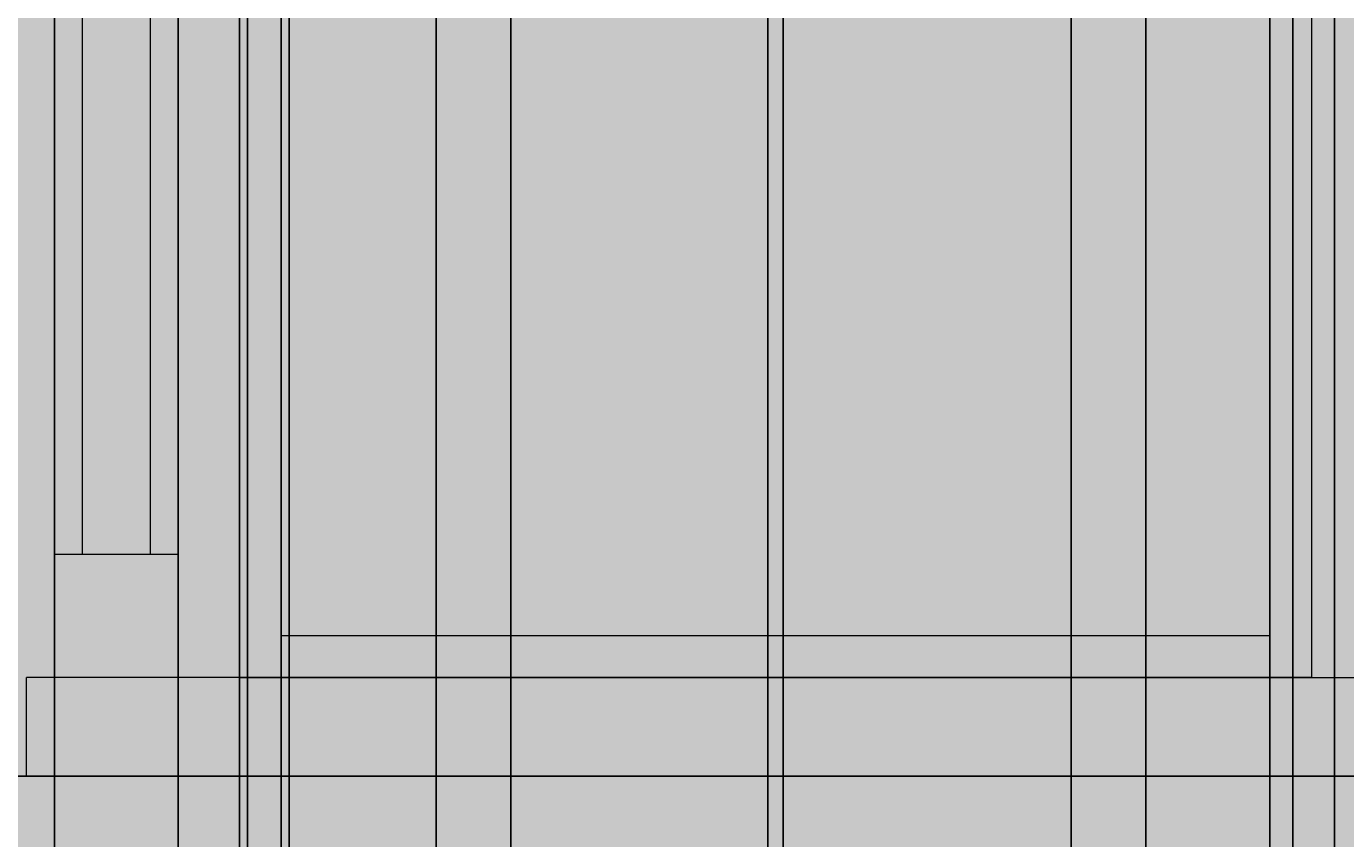
# Model space of a CAD drawing. Units: inches. Extents: x 3024 to 4744, y 1110 to 2100.
# Tile 19 of 29: x 3149 to 3275, y 1654 to 1731. Entities that reach past the tile are written whole.
import ezdxf

# ---------------------------------------------------------------- set-up
doc = ezdxf.new("R2010")
doc.units = ezdxf.units.IN
for name, color, linetype, lineweight in [('A-ANNO-DIMS', 2, 'Continuous', 18), ('A-ELEV', 7, 'Continuous', 25), ('A-ELEV-PATT', 252, 'Continuous', 13), ('A-GLAZ', 4, 'Continuous', 18)]:
    doc.layers.add(name, color=color, linetype=linetype, lineweight=lineweight)
doc.styles.get("Standard").update_dxf_attribs({"font": 'arial.ttf'})
doc.dimstyles.get("Standard").update_dxf_attribs({"dimtxt": 0.18, "dimasz": 0.18, "dimexe": 0.18, "dimexo": 0.0625, "dimgap": 0.09, "dimtad": 0, "dimtih": 1, "dimtoh": 1, "dimdec": 1, "dimzin": 0, "dimdsep": 46, "dimlunit": 3, "dimtxsty": 'Standard', "dimcen": 0.09, "dimadec": 0, "dimazin": 0, "dimtfac": 1, "dimtdec": 1, "dimtofl": 0, "dimtmove": 0, "dimatfit": 3, "dimfxl": 1, "dimtolj": 1, "dimtzin": 0, "dimarcsym": 0})

# ---------------------------------------------------------------- blocks, each defined once
blk = doc.blocks.new('WIN-BALCONY-A')
for q in [(3148.97, 1795.04), (3148.97, 1795.04), (3292.61, 1795.04), (3292.61, 1795.04)]:
    blk.add_line((3169.4, 1795.04), q)
for points in [[(3154.33, 1806.87), (3160.86, 1806.87), (3160.86, 1897.49), (3154.33, 1897.49)], [(3154.33, 1806.87), (3160.86, 1806.87), (3160.86, 1897.49), (3154.33, 1897.49)], [(3272.18, 1795.04), (3169.4, 1795.04), (3169.4, 1897.49), (3272.18, 1897.49)], [(3272.18, 1795.04), (3169.4, 1795.04), (3169.4, 1897.49), (3272.18, 1897.49)], [(3268.18, 1799.04), (3173.4, 1799.04), (3173.4, 1893.49), (3268.18, 1893.49)], [(3268.18, 1799.04), (3173.4, 1799.04), (3173.4, 1893.49), (3268.18, 1893.49)], [(3220.05, 1893.49), (3221.52, 1893.49), (3221.52, 1799.04), (3220.05, 1799.04)], [(3220.05, 1893.49), (3221.52, 1893.49), (3221.52, 1799.04), (3220.05, 1799.04)], [(3163.53, 1795.04), (3151.66, 1795.04), (3151.66, 1806.87), (3163.53, 1806.87)], [(3163.53, 1795.04), (3151.66, 1795.04), (3151.66, 1806.87), (3163.53, 1806.87)]]:
    blk.add_lwpolyline(points, close=True)
blk.add_lwpolyline([(3292.61, 1795.04), (3292.61, 1785.61), (3148.97, 1785.61), (3148.97, 1795.04)])
blk.add_lwpolyline([(3292.61, 1795.04), (3292.61, 1785.61), (3148.97, 1785.61), (3148.97, 1795.04)])
blk = doc.blocks.new('*D64')
at = {"layer": 'A-ANNO-DIMS', "color": 0, "lineweight": -2, "transparency": 16777216}
for p, q in [((3069.79, 1241.5), (3069.79, 2100.44)), ((3069.97, 2100.26), (3405.08, 2100.26)), ((3740.97, 2100.26), (3405.87, 2100.26)), ((3741.15, 1241.5), (3741.15, 2100.44))]:
    blk.add_line(p, q, dxfattribs=at)
at = {"layer": 'A-ANNO-DIMS', "color": 0, "transparency": 16777216}
for points in [[(3069.97, 2100.29), (3069.97, 2100.23), (3069.79, 2100.26)], [(3740.97, 2100.29), (3740.97, 2100.23), (3741.15, 2100.26)]]:
    blk.add_solid(points, dxfattribs=at)
at = {"layer": 'Defpoints', "color": 0, "transparency": 16777216}
for p in [(3741.15, 2100.26), (3069.79, 1241.43), (3741.15, 1241.43)]:
    blk.add_point(p, dxfattribs=at)
at = {"layer": 'A-ANNO-DIMS', "color": 0, "transparency": 16777216, "insert": (3405.47, 2100.26), "char_height": 0.18, "attachment_point": 5}
blk.add_mtext('\\A1;671.4', dxfattribs=at)
blk = doc.blocks.new('*D89')
at = {"layer": 'A-ANNO-DIMS', "color": 0, "lineweight": -2, "transparency": 16777216}
for p, q in [((3151.66, 1794.98), (3151.66, 1109.93)), ((3163.53, 1794.98), (3163.53, 1109.93)), ((3151.84, 1110.11), (3157.14, 1110.11)), ((3163.35, 1110.11), (3158.05, 1110.11))]:
    blk.add_line(p, q, dxfattribs=at)
at = {"layer": 'A-ANNO-DIMS', "color": 0, "transparency": 16777216}
for points in [[(3151.84, 1110.14), (3151.84, 1110.08), (3151.66, 1110.11)], [(3163.35, 1110.14), (3163.35, 1110.08), (3163.53, 1110.11)]]:
    blk.add_solid(points, dxfattribs=at)
at = {"layer": 'Defpoints', "color": 0, "transparency": 16777216}
for p in [(3151.66, 1795.04), (3163.53, 1795.04), (3163.53, 1110.11)]:
    blk.add_point(p, dxfattribs=at)
at = {"layer": 'A-ANNO-DIMS', "color": 0, "transparency": 16777216, "insert": (3157.59, 1110.11), "char_height": 0.18, "attachment_point": 5}
blk.add_mtext('\\A1;11.866', dxfattribs=at)
blk = doc.blocks.new('*D90')
at = {"layer": 'A-ANNO-DIMS', "color": 0, "lineweight": -2, "transparency": 16777216}
for p, q in [((3173.4, 1798.98), (3173.4, 1109.93)), ((3169.4, 1794.98), (3169.4, 1109.93)), ((3169.58, 1110.11), (3171.07, 1110.11)), ((3173.22, 1110.11), (3171.72, 1110.11))]:
    blk.add_line(p, q, dxfattribs=at)
at = {"layer": 'A-ANNO-DIMS', "color": 0, "transparency": 16777216}
for points in [[(3169.58, 1110.14), (3169.58, 1110.08), (3169.4, 1110.11)], [(3173.22, 1110.14), (3173.22, 1110.08), (3173.4, 1110.11)]]:
    blk.add_solid(points, dxfattribs=at)
at = {"layer": 'Defpoints', "color": 0, "transparency": 16777216}
for p in [(3173.4, 1799.04), (3169.4, 1795.04), (3173.4, 1110.11)]:
    blk.add_point(p, dxfattribs=at)
at = {"layer": 'A-ANNO-DIMS', "color": 0, "transparency": 16777216, "insert": (3171.4, 1110.11), "char_height": 0.18, "attachment_point": 5}
blk.add_mtext('\\A1;4.00', dxfattribs=at)
blk = doc.blocks.new('*D91')
at = {"layer": 'A-ANNO-DIMS', "color": 0, "lineweight": -2, "transparency": 16777216}
for p, q in [((3173.4, 1798.98), (3173.4, 1109.93)), ((3220.05, 1798.98), (3220.05, 1109.93)), ((3173.58, 1110.11), (3196.33, 1110.11)), ((3219.87, 1110.11), (3197.12, 1110.11))]:
    blk.add_line(p, q, dxfattribs=at)
at = {"layer": 'A-ANNO-DIMS', "color": 0, "transparency": 16777216}
for points in [[(3173.58, 1110.14), (3173.58, 1110.08), (3173.4, 1110.11)], [(3219.87, 1110.14), (3219.87, 1110.08), (3220.05, 1110.11)]]:
    blk.add_solid(points, dxfattribs=at)
at = {"layer": 'Defpoints', "color": 0, "transparency": 16777216}
for p in [(3173.4, 1799.04), (3220.05, 1799.04), (3220.05, 1110.11)]:
    blk.add_point(p, dxfattribs=at)
at = {"layer": 'A-ANNO-DIMS', "color": 0, "transparency": 16777216, "insert": (3196.72, 1110.11), "char_height": 0.18, "attachment_point": 5}
blk.add_mtext('\\A1;46.65', dxfattribs=at)
blk = doc.blocks.new('*D92')
at = {"layer": 'A-ANNO-DIMS', "color": 0, "lineweight": -2, "transparency": 16777216}
for p, q in [((3220.05, 1798.98), (3220.05, 1109.93)), ((3221.52, 1798.98), (3221.52, 1109.93)), ((3220.23, 1110.11), (3220.47, 1110.11)), ((3221.34, 1110.11), (3221.1, 1110.11))]:
    blk.add_line(p, q, dxfattribs=at)
at = {"layer": 'A-ANNO-DIMS', "color": 0, "transparency": 16777216}
for points in [[(3220.23, 1110.14), (3220.23, 1110.08), (3220.05, 1110.11)], [(3221.34, 1110.14), (3221.34, 1110.08), (3221.52, 1110.11)]]:
    blk.add_solid(points, dxfattribs=at)
at = {"layer": 'Defpoints', "color": 0, "transparency": 16777216}
for p in [(3220.05, 1799.04), (3221.52, 1799.04), (3221.52, 1110.11)]:
    blk.add_point(p, dxfattribs=at)
at = {"layer": 'A-ANNO-DIMS', "color": 0, "transparency": 16777216, "insert": (3220.79, 1110.11), "char_height": 0.18, "attachment_point": 5}
blk.add_mtext('\\A1;1.47', dxfattribs=at)
blk = doc.blocks.new('*D93')
at = {"layer": 'A-ANNO-DIMS', "color": 0, "lineweight": -2, "transparency": 16777216}
for p, q in [((3221.52, 1798.98), (3221.52, 1109.93)), ((3268.18, 1798.98), (3268.18, 1109.93)), ((3221.7, 1110.11), (3244.45, 1110.11)), ((3268, 1110.11), (3245.25, 1110.11))]:
    blk.add_line(p, q, dxfattribs=at)
at = {"layer": 'A-ANNO-DIMS', "color": 0, "transparency": 16777216}
for points in [[(3221.7, 1110.14), (3221.7, 1110.08), (3221.52, 1110.11)], [(3268, 1110.14), (3268, 1110.08), (3268.18, 1110.11)]]:
    blk.add_solid(points, dxfattribs=at)
at = {"layer": 'Defpoints', "color": 0, "transparency": 16777216}
for p in [(3221.52, 1799.04), (3268.18, 1799.04), (3268.18, 1110.11)]:
    blk.add_point(p, dxfattribs=at)
at = {"layer": 'A-ANNO-DIMS', "color": 0, "transparency": 16777216, "insert": (3244.85, 1110.11), "char_height": 0.18, "attachment_point": 5}
blk.add_mtext('\\A1;46.65', dxfattribs=at)
blk = doc.blocks.new('*D106')
at = {"layer": 'A-ANNO-DIMS', "color": 0, "lineweight": -2, "transparency": 16777216}
for p, q in [((3170.16, 1275.67), (3170.16, 2100.44)), ((3170.34, 2100.26), (3171.83, 2100.26)), ((3173.98, 2100.26), (3172.49, 2100.26)), ((3174.16, 1271.67), (3174.16, 2100.44))]:
    blk.add_line(p, q, dxfattribs=at)
at = {"layer": 'A-ANNO-DIMS', "color": 0, "transparency": 16777216}
for points in [[(3170.34, 2100.29), (3170.34, 2100.23), (3170.16, 2100.26)], [(3173.98, 2100.29), (3173.98, 2100.23), (3174.16, 2100.26)]]:
    blk.add_solid(points, dxfattribs=at)
at = {"layer": 'Defpoints', "color": 0, "transparency": 16777216}
for p in [(3174.16, 2100.26), (3170.16, 1275.61), (3174.16, 1271.61)]:
    blk.add_point(p, dxfattribs=at)
at = {"layer": 'A-ANNO-DIMS', "color": 0, "transparency": 16777216, "insert": (3172.16, 2100.26), "char_height": 0.18, "attachment_point": 5}
blk.add_mtext('\\A1;4.00', dxfattribs=at)
blk = doc.blocks.new('*D107')
at = {"layer": 'A-ANNO-DIMS', "color": 0, "lineweight": -2, "transparency": 16777216}
for p, q in [((3174.16, 1271.67), (3174.16, 2100.44)), ((3174.34, 2100.26), (3221.88, 2100.26)), ((3270.21, 2100.26), (3222.67, 2100.26)), ((3270.39, 1271.67), (3270.39, 2100.44))]:
    blk.add_line(p, q, dxfattribs=at)
at = {"layer": 'A-ANNO-DIMS', "color": 0, "transparency": 16777216}
for points in [[(3174.34, 2100.29), (3174.34, 2100.23), (3174.16, 2100.26)], [(3270.21, 2100.29), (3270.21, 2100.23), (3270.39, 2100.26)]]:
    blk.add_solid(points, dxfattribs=at)
at = {"layer": 'Defpoints', "color": 0, "transparency": 16777216}
for p in [(3270.39, 2100.26), (3174.16, 1271.61), (3270.39, 1271.61)]:
    blk.add_point(p, dxfattribs=at)
at = {"layer": 'A-ANNO-DIMS', "color": 0, "transparency": 16777216, "insert": (3222.27, 2100.26), "char_height": 0.18, "attachment_point": 5}
blk.add_mtext('\\A1;96.23', dxfattribs=at)
blk = doc.blocks.new('*D108')
at = {"layer": 'A-ANNO-DIMS', "color": 0, "lineweight": -2, "transparency": 16777216}
for p, q in [((3270.39, 1271.67), (3270.39, 2100.44)), ((3270.57, 2100.26), (3272.06, 2100.26)), ((3274.21, 2100.26), (3272.71, 2100.26)), ((3274.39, 1275.67), (3274.39, 2100.44))]:
    blk.add_line(p, q, dxfattribs=at)
at = {"layer": 'A-ANNO-DIMS', "color": 0, "transparency": 16777216}
for points in [[(3270.57, 2100.29), (3270.57, 2100.23), (3270.39, 2100.26)], [(3274.21, 2100.29), (3274.21, 2100.23), (3274.39, 2100.26)]]:
    blk.add_solid(points, dxfattribs=at)
at = {"layer": 'Defpoints', "color": 0, "transparency": 16777216}
for p in [(3274.39, 2100.26), (3274.39, 1275.61), (3270.39, 1271.61)]:
    blk.add_point(p, dxfattribs=at)
at = {"layer": 'A-ANNO-DIMS', "color": 0, "transparency": 16777216, "insert": (3272.39, 2100.26), "char_height": 0.18, "attachment_point": 5}
blk.add_mtext('\\A1;4.00', dxfattribs=at)
blk = doc.blocks.new('*D124')
at = {"layer": 'A-ANNO-DIMS', "color": 0, "lineweight": -2, "transparency": 16777216}
for p, q in [((3174.16, 1271.67), (3174.16, 2100.44)), ((3174.34, 2100.26), (3180.75, 2100.26)), ((3188.08, 2100.26), (3181.67, 2100.26)), ((3188.26, 1256.29), (3188.26, 2100.44))]:
    blk.add_line(p, q, dxfattribs=at)
at = {"layer": 'A-ANNO-DIMS', "color": 0, "transparency": 16777216}
for points in [[(3174.34, 2100.29), (3174.34, 2100.23), (3174.16, 2100.26)], [(3188.08, 2100.29), (3188.08, 2100.23), (3188.26, 2100.26)]]:
    blk.add_solid(points, dxfattribs=at)
at = {"layer": 'Defpoints', "color": 0, "transparency": 16777216}
for p in [(3188.26, 2100.26), (3174.16, 1271.61), (3188.26, 1256.23)]:
    blk.add_point(p, dxfattribs=at)
at = {"layer": 'A-ANNO-DIMS', "color": 0, "transparency": 16777216, "insert": (3181.21, 2100.26), "char_height": 0.18, "attachment_point": 5}
blk.add_mtext('\\A1;14.098', dxfattribs=at)
blk = doc.blocks.new('*D125')
at = {"layer": 'A-ANNO-DIMS', "color": 0, "lineweight": -2, "transparency": 16777216}
for p, q in [((3188.26, 1256.29), (3188.26, 2100.44)), ((3188.44, 2100.26), (3191.44, 2100.26)), ((3195.23, 2100.26), (3192.22, 2100.26)), ((3195.41, 1256.29), (3195.41, 2100.44))]:
    blk.add_line(p, q, dxfattribs=at)
at = {"layer": 'A-ANNO-DIMS', "color": 0, "transparency": 16777216}
for points in [[(3188.44, 2100.29), (3188.44, 2100.23), (3188.26, 2100.26)], [(3195.23, 2100.29), (3195.23, 2100.23), (3195.41, 2100.26)]]:
    blk.add_solid(points, dxfattribs=at)
at = {"layer": 'Defpoints', "color": 0, "transparency": 16777216}
for p in [(3195.41, 2100.26), (3188.26, 1256.23), (3195.41, 1256.23)]:
    blk.add_point(p, dxfattribs=at)
at = {"layer": 'A-ANNO-DIMS', "color": 0, "transparency": 16777216, "insert": (3191.83, 2100.26), "char_height": 0.18, "attachment_point": 5}
blk.add_mtext('\\A1;7.147', dxfattribs=at)
blk = doc.blocks.new('*D126')
at = {"layer": 'A-ANNO-DIMS', "color": 0, "lineweight": -2, "transparency": 16777216}
for p, q in [((3249.14, 1256.29), (3249.14, 2100.44)), ((3249.32, 2100.26), (3252.32, 2100.26)), ((3256.11, 2100.26), (3253.11, 2100.26)), ((3256.29, 1256.29), (3256.29, 2100.44))]:
    blk.add_line(p, q, dxfattribs=at)
at = {"layer": 'A-ANNO-DIMS', "color": 0, "transparency": 16777216}
for points in [[(3249.32, 2100.29), (3249.32, 2100.23), (3249.14, 2100.26)], [(3256.11, 2100.29), (3256.11, 2100.23), (3256.29, 2100.26)]]:
    blk.add_solid(points, dxfattribs=at)
at = {"layer": 'Defpoints', "color": 0, "transparency": 16777216}
for p in [(3256.29, 2100.26), (3249.14, 1256.23), (3256.29, 1256.23)]:
    blk.add_point(p, dxfattribs=at)
at = {"layer": 'A-ANNO-DIMS', "color": 0, "transparency": 16777216, "insert": (3252.72, 2100.26), "char_height": 0.18, "attachment_point": 5}
blk.add_mtext('\\A1;7.147', dxfattribs=at)

msp = doc.modelspace()

# ---------------------------------------------------------------- hatches: boundary and pattern name
at = {"layer": 'A-ELEV-PATT'}
h = msp.add_hatch(color=256, dxfattribs=at)
h.dxf.hatch_style = 1
h.paths.add_polyline_path([(3491.8271, 2054.7584), (3320.5658, 2054.7584), (3320.5658, 2043.5286), (3491.8271, 2043.5286)])
h.paths.add_polyline_path([(3292.6051, 1905.6112), (3148.9694, 1905.6112), (3148.9694, 1897.4879), (3169.3964, 1897.4879), (3292.6051, 1897.4879)])
h.paths.add_polyline_path([(3292.6051, 1795.0431), (3169.3964, 1795.0431), (3148.9694, 1795.0431), (3148.9694, 1785.6112), (3292.6051, 1785.6112)])
h.paths.add_polyline_path([(3292.6051, 1779.6112), (3148.9694, 1779.6112), (3148.9694, 1771.4879), (3169.3964, 1771.4879), (3292.6051, 1771.4879)])
h.paths.add_polyline_path([(3292.6051, 1669.0431), (3169.3964, 1669.0431), (3148.9694, 1669.0431), (3148.9694, 1659.6112), (3292.6051, 1659.6112)])
h.paths.add_polyline_path([(3292.6051, 1653.6112), (3148.9694, 1653.6112), (3148.9694, 1645.4879), (3169.3964, 1645.4879), (3292.6051, 1645.4879)])
h.paths.add_polyline_path([(3292.6051, 1543.0431), (3169.3964, 1543.0431), (3148.9694, 1543.0431), (3148.9694, 1533.6112), (3292.6051, 1533.6112)])
h.paths.add_polyline_path([(3292.6051, 1527.6112), (3148.9694, 1527.6112), (3148.9694, 1519.4879), (3169.3964, 1519.4879), (3292.6051, 1519.4879)])
h.paths.add_polyline_path([(3292.6051, 1401.6112), (3148.9694, 1401.6112), (3148.9694, 1393.4879), (3169.3964, 1393.4879), (3292.6051, 1393.4879)])
h.paths.add_polyline_path([(3292.6051, 1417.0431), (3169.3964, 1417.0431), (3148.9694, 1417.0431), (3148.9694, 1407.6112), (3292.6051, 1407.6112)])
h.paths.add_polyline_path([(3292.6051, 1291.0431), (3169.3964, 1291.0431), (3148.9694, 1291.0431), (3148.9694, 1281.6112), (3292.6051, 1281.6112)])
h.paths.add_polyline_path([(3654.037, 1165.0431), (3530.8283, 1165.0431), (3510.4013, 1165.0431), (3510.4013, 1155.6112), (3654.037, 1155.6112)])
h.paths.add_polyline_path([(3654.037, 1275.6112), (3510.4013, 1275.6112), (3510.4013, 1267.4879), (3530.8283, 1267.4879), (3654.037, 1267.4879)])
h.paths.add_polyline_path([(3654.037, 1291.0431), (3530.8283, 1291.0431), (3510.4013, 1291.0431), (3510.4013, 1281.6112), (3654.037, 1281.6112)])
h.paths.add_polyline_path([(3654.037, 1417.0431), (3530.8283, 1417.0431), (3510.4013, 1417.0431), (3510.4013, 1407.6112), (3654.037, 1407.6112)])
h.paths.add_polyline_path([(3654.037, 1401.6112), (3510.4013, 1401.6112), (3510.4013, 1393.4879), (3530.8283, 1393.4879), (3654.037, 1393.4879)])
h.paths.add_polyline_path([(3654.037, 1543.0431), (3530.8283, 1543.0431), (3510.4013, 1543.0431), (3510.4013, 1533.6112), (3654.037, 1533.6112)])
h.paths.add_polyline_path([(3654.037, 1527.6112), (3510.4013, 1527.6112), (3510.4013, 1519.4879), (3530.8283, 1519.4879), (3654.037, 1519.4879)])
h.paths.add_polyline_path([(3654.037, 1653.6112), (3510.4013, 1653.6112), (3510.4013, 1645.4879), (3530.8283, 1645.4879), (3654.037, 1645.4879)])
h.paths.add_polyline_path([(3654.037, 1669.0431), (3530.8283, 1669.0431), (3510.4013, 1669.0431), (3510.4013, 1659.6112), (3654.037, 1659.6112)])
h.paths.add_polyline_path([(3654.037, 1779.6112), (3510.4013, 1779.6112), (3510.4013, 1771.4879), (3530.8283, 1771.4879), (3654.037, 1771.4879)])
h.paths.add_polyline_path([(3654.037, 1795.0431), (3530.8283, 1795.0431), (3510.4013, 1795.0431), (3510.4013, 1785.6112), (3654.037, 1785.6112)])
h.paths.add_polyline_path([(3654.037, 1905.6112), (3510.4013, 1905.6112), (3510.4013, 1897.4879), (3530.8283, 1897.4879), (3654.037, 1897.4879)])
h = msp.add_hatch(color=256, dxfattribs=at)
h.dxf.hatch_style = 1
h.paths.add_polyline_path([(3329.7033, 1407.6112), (3105.4722, 1407.6112), (3105.4722, 1401.6112), (3329.7033, 1401.6112)])
h.paths.add_polyline_path([(3329.7033, 1281.6112), (3105.4722, 1281.6112), (3105.4722, 1275.6112), (3112.3838, 1275.6112), (3329.7033, 1275.6112)])
h.paths.add_polyline_path([(3329.7033, 1533.6112), (3105.4722, 1533.6112), (3105.4722, 1527.6112), (3329.7033, 1527.6112)])
h.paths.add_polyline_path([(3329.7033, 1659.6112), (3105.4722, 1659.6112), (3105.4722, 1653.6112), (3329.7033, 1653.6112)])
h.paths.add_polyline_path([(3329.7033, 1785.6112), (3105.4722, 1785.6112), (3105.4722, 1779.6112), (3329.7033, 1779.6112)])
h.paths.add_polyline_path([(3329.7033, 1911.6112), (3105.4722, 1911.6112), (3095.7158, 1911.6112), (3095.7158, 1905.6112), (3329.7033, 1905.6112)])
h.paths.add_polyline_path([(3715.2286, 1911.6112), (3705.4722, 1911.6112), (3705.4722, 1905.6112), (3715.2286, 1905.6112)])
h.paths.add_polyline_path([(3688.5588, 1911.6112), (3481.2411, 1911.6112), (3481.2411, 1905.6112), (3688.5588, 1905.6112)])
h = msp.add_hatch(color=256, dxfattribs=at)
h.dxf.hatch_style = 1
h.paths.add_polyline_path([(3154.3287, 1897.4879), (3148.9694, 1897.4879), (3148.9694, 1905.6112), (3105.4722, 1905.6112), (3105.4722, 1785.6112), (3148.9694, 1785.6112), (3148.9694, 1795.0431), (3151.6604, 1795.0431), (3151.6604, 1806.8674), (3154.3287, 1806.8674)])
h.paths.add_polyline_path([(3329.7033, 1905.6112), (3292.6051, 1905.6112), (3292.6051, 1897.4879), (3287.2458, 1897.4879), (3287.2458, 1806.8674), (3288.3759, 1806.8674), (3288.3759, 1795.0431), (3292.6051, 1795.0431), (3292.6051, 1785.6112), (3329.7033, 1785.6112)])
h.paths.add_polyline_path([(3154.3287, 1771.4879), (3148.9694, 1771.4879), (3148.9694, 1779.6112), (3105.4722, 1779.6112), (3105.4722, 1659.6112), (3148.9694, 1659.6112), (3148.9694, 1669.0431), (3151.6604, 1669.0431), (3151.6604, 1680.8674), (3154.3287, 1680.8674)])
h.paths.add_polyline_path([(3329.7033, 1779.6112), (3292.6051, 1779.6112), (3292.6051, 1771.4879), (3287.2458, 1771.4879), (3287.2458, 1680.8674), (3288.3759, 1680.8674), (3288.3759, 1669.0431), (3292.6051, 1669.0431), (3292.6051, 1659.6112), (3329.7033, 1659.6112)])
h.paths.add_polyline_path([(3154.3287, 1645.4879), (3148.9694, 1645.4879), (3148.9694, 1653.6112), (3105.4722, 1653.6112), (3105.4722, 1533.6112), (3148.9694, 1533.6112), (3148.9694, 1543.0431), (3151.6604, 1543.0431), (3151.6604, 1554.8674), (3154.3287, 1554.8674)])
h.paths.add_polyline_path([(3329.7033, 1653.6112), (3292.6051, 1653.6112), (3292.6051, 1645.4879), (3287.2458, 1645.4879), (3287.2458, 1554.8674), (3288.3759, 1554.8674), (3288.3759, 1543.0431), (3292.6051, 1543.0431), (3292.6051, 1533.6112), (3329.7033, 1533.6112)])
h.paths.add_polyline_path([(3329.7033, 1527.6112), (3292.6051, 1527.6112), (3292.6051, 1519.4879), (3287.2458, 1519.4879), (3287.2458, 1428.8674), (3288.3759, 1428.8674), (3288.3759, 1417.0431), (3292.6051, 1417.0431), (3292.6051, 1407.6112), (3329.7033, 1407.6112)])
h.paths.add_polyline_path([(3329.7033, 1401.6112), (3292.6051, 1401.6112), (3292.6051, 1393.4879), (3287.2458, 1393.4879), (3287.2458, 1302.8674), (3288.3759, 1302.8674), (3288.3759, 1291.0431), (3292.6051, 1291.0431), (3292.6051, 1281.6112), (3329.7033, 1281.6112)])
h.paths.add_polyline_path([(3154.3287, 1393.4879), (3148.9694, 1393.4879), (3148.9694, 1401.6112), (3105.4722, 1401.6112), (3105.4722, 1281.6112), (3148.9694, 1281.6112), (3148.9694, 1291.0431), (3151.6604, 1291.0431), (3151.6604, 1302.8674), (3154.3287, 1302.8674)])
h.paths.add_polyline_path([(3154.3287, 1519.4879), (3148.9694, 1519.4879), (3148.9694, 1527.6112), (3105.4722, 1527.6112), (3105.4722, 1407.6112), (3148.9694, 1407.6112), (3148.9694, 1417.0431), (3151.6604, 1417.0431), (3151.6604, 1428.8674), (3154.3287, 1428.8674)])
h.paths.add_polyline_path([(3515.7606, 1897.4879), (3510.4013, 1897.4879), (3510.4013, 1905.6112), (3481.2411, 1905.6112), (3481.2411, 1785.6112), (3510.4013, 1785.6112), (3510.4013, 1795.0431), (3513.0923, 1795.0431), (3513.0923, 1806.8674), (3515.7606, 1806.8674)])
h.paths.add_polyline_path([(3688.5588, 1905.6112), (3654.037, 1905.6112), (3654.037, 1897.4879), (3648.6777, 1897.4879), (3648.6777, 1806.8674), (3649.8078, 1806.8674), (3649.8078, 1795.0431), (3654.037, 1795.0431), (3654.037, 1785.6112), (3688.5588, 1785.6112)])
h.paths.add_polyline_path([(3515.7606, 1771.4879), (3510.4013, 1771.4879), (3510.4013, 1779.6112), (3481.2411, 1779.6112), (3481.2411, 1659.6112), (3510.4013, 1659.6112), (3510.4013, 1669.0431), (3513.0923, 1669.0431), (3513.0923, 1680.8674), (3515.7606, 1680.8674)])
h.paths.add_polyline_path([(3688.5588, 1779.6112), (3654.037, 1779.6112), (3654.037, 1771.4879), (3648.6777, 1771.4879), (3648.6777, 1680.8674), (3649.8078, 1680.8674), (3649.8078, 1669.0431), (3654.037, 1669.0431), (3654.037, 1659.6112), (3688.5588, 1659.6112)])
h.paths.add_polyline_path([(3515.7606, 1645.4879), (3510.4013, 1645.4879), (3510.4013, 1653.6112), (3481.2411, 1653.6112), (3481.2411, 1533.6112), (3510.4013, 1533.6112), (3510.4013, 1543.0431), (3513.0923, 1543.0431), (3513.0923, 1554.8674), (3515.7606, 1554.8674)])
h.paths.add_polyline_path([(3688.5588, 1653.6112), (3654.037, 1653.6112), (3654.037, 1645.4879), (3648.6777, 1645.4879), (3648.6777, 1554.8674), (3649.8078, 1554.8674), (3649.8078, 1543.0431), (3654.037, 1543.0431), (3654.037, 1533.6112), (3688.5588, 1533.6112)])
h.paths.add_polyline_path([(3515.7606, 1519.4879), (3510.4013, 1519.4879), (3510.4013, 1527.6112), (3481.2411, 1527.6112), (3481.2411, 1407.6112), (3510.4013, 1407.6112), (3510.4013, 1417.0431), (3513.0923, 1417.0431), (3513.0923, 1428.8674), (3515.7606, 1428.8674)])
h.paths.add_polyline_path([(3688.5588, 1527.6112), (3654.037, 1527.6112), (3654.037, 1519.4879), (3648.6777, 1519.4879), (3648.6777, 1428.8674), (3649.8078, 1428.8674), (3649.8078, 1417.0431), (3654.037, 1417.0431), (3654.037, 1407.6112), (3688.5588, 1407.6112)])
h.paths.add_polyline_path([(3515.7606, 1393.4879), (3510.4013, 1393.4879), (3510.4013, 1401.6112), (3481.2411, 1401.6112), (3481.2411, 1281.6112), (3510.4013, 1281.6112), (3510.4013, 1291.0431), (3513.0923, 1291.0431), (3513.0923, 1302.8674), (3515.7606, 1302.8674)])
h.paths.add_polyline_path([(3688.5588, 1401.6112), (3654.037, 1401.6112), (3654.037, 1393.4879), (3648.6777, 1393.4879), (3648.6777, 1302.8674), (3649.8078, 1302.8674), (3649.8078, 1291.0431), (3654.037, 1291.0431), (3654.037, 1281.6112), (3688.5588, 1281.6112)])
h.paths.add_polyline_path([(3515.7606, 1267.4879), (3510.4013, 1267.4879), (3510.4013, 1275.6112), (3481.2411, 1275.6112), (3481.2411, 1155.6112), (3510.4013, 1155.6112), (3510.4013, 1165.0431), (3513.0923, 1165.0431), (3513.0923, 1176.8674), (3515.7606, 1176.8674)])
h.paths.add_polyline_path([(3688.5588, 1275.6112), (3654.037, 1275.6112), (3654.037, 1267.4879), (3648.6777, 1267.4879), (3648.6777, 1176.8674), (3649.8078, 1176.8674), (3649.8078, 1165.0431), (3654.037, 1165.0431), (3654.037, 1155.6112), (3688.5588, 1155.6112)])
h.paths.add_polyline_path([(3112.3838, 1275.6112), (3105.4722, 1275.6112), (3105.4722, 1171.0239), (3112.3838, 1171.0239)])
h = msp.add_hatch(color=256, dxfattribs=at)
h.dxf.hatch_style = 1
h.paths.add_polyline_path([(3160.8586, 1897.4879), (3154.3287, 1897.4879), (3154.3287, 1806.8674), (3160.8586, 1806.8674)])
h.paths.add_polyline_path([(3287.2458, 1897.4879), (3280.716, 1897.4879), (3280.716, 1806.8674), (3287.2458, 1806.8674)])
h.paths.add_polyline_path([(3160.8586, 1771.4879), (3154.3287, 1771.4879), (3154.3287, 1680.8674), (3160.8586, 1680.8674)])
h.paths.add_polyline_path([(3287.2458, 1771.4879), (3280.716, 1771.4879), (3280.716, 1680.8674), (3287.2458, 1680.8674)])
h.paths.add_polyline_path([(3160.8586, 1645.4879), (3154.3287, 1645.4879), (3154.3287, 1554.8674), (3160.8586, 1554.8674)])
h.paths.add_polyline_path([(3287.2458, 1645.4879), (3280.716, 1645.4879), (3280.716, 1554.8674), (3287.2458, 1554.8674)])
h.paths.add_polyline_path([(3160.8586, 1519.4879), (3154.3287, 1519.4879), (3154.3287, 1428.8674), (3160.8586, 1428.8674)])
h.paths.add_polyline_path([(3287.2458, 1519.4879), (3280.716, 1519.4879), (3280.716, 1428.8674), (3287.2458, 1428.8674)])
h.paths.add_polyline_path([(3160.8586, 1393.4879), (3154.3287, 1393.4879), (3154.3287, 1302.8674), (3160.8586, 1302.8674)])
h.paths.add_polyline_path([(3287.2458, 1393.4879), (3280.716, 1393.4879), (3280.716, 1302.8674), (3287.2458, 1302.8674)])
h.paths.add_polyline_path([(3648.6777, 1267.4879), (3642.1479, 1267.4879), (3642.1479, 1176.8674), (3648.6777, 1176.8674)])
h.paths.add_polyline_path([(3522.2905, 1267.4879), (3515.7606, 1267.4879), (3515.7606, 1176.8674), (3522.2905, 1176.8674)])
h.paths.add_polyline_path([(3522.2905, 1393.4879), (3515.7606, 1393.4879), (3515.7606, 1302.8674), (3522.2905, 1302.8674)])
h.paths.add_polyline_path([(3648.6777, 1393.4879), (3642.1479, 1393.4879), (3642.1479, 1302.8674), (3648.6777, 1302.8674)])
h.paths.add_polyline_path([(3522.2905, 1519.4879), (3515.7606, 1519.4879), (3515.7606, 1428.8674), (3522.2905, 1428.8674)])
h.paths.add_polyline_path([(3648.6777, 1519.4879), (3642.1479, 1519.4879), (3642.1479, 1428.8674), (3648.6777, 1428.8674)])
h.paths.add_polyline_path([(3522.2905, 1645.4879), (3515.7606, 1645.4879), (3515.7606, 1554.8674), (3522.2905, 1554.8674)])
h.paths.add_polyline_path([(3522.2905, 1771.4879), (3515.7606, 1771.4879), (3515.7606, 1680.8674), (3522.2905, 1680.8674)])
h.paths.add_polyline_path([(3648.6777, 1645.4879), (3642.1479, 1645.4879), (3642.1479, 1554.8674), (3648.6777, 1554.8674)])
h.paths.add_polyline_path([(3648.6777, 1771.4879), (3642.1479, 1771.4879), (3642.1479, 1680.8674), (3648.6777, 1680.8674)])
h.paths.add_polyline_path([(3648.6777, 1897.4879), (3642.1479, 1897.4879), (3642.1479, 1806.8674), (3648.6777, 1806.8674)])
h.paths.add_polyline_path([(3522.2905, 1897.4879), (3515.7606, 1897.4879), (3515.7606, 1806.8674), (3522.2905, 1806.8674)])
h = msp.add_hatch(color=256, dxfattribs=at)
h.dxf.hatch_style = 1
h.paths.add_polyline_path([(3169.3964, 1897.4879), (3160.8586, 1897.4879), (3160.8586, 1806.8674), (3163.5269, 1806.8674), (3163.5269, 1795.0431), (3169.3964, 1795.0431)])
h.paths.add_polyline_path([(3280.716, 1897.4879), (3272.1781, 1897.4879), (3272.1781, 1795.0431), (3276.5094, 1795.0431), (3276.5094, 1806.8674), (3280.716, 1806.8674)])
h.paths.add_polyline_path([(3280.716, 1771.4879), (3272.1781, 1771.4879), (3272.1781, 1669.0431), (3276.5094, 1669.0431), (3276.5094, 1680.8674), (3280.716, 1680.8674)])
h.paths.add_polyline_path([(3169.3964, 1771.4879), (3160.8586, 1771.4879), (3160.8586, 1680.8674), (3163.5269, 1680.8674), (3163.5269, 1669.0431), (3169.3964, 1669.0431)])
h.paths.add_polyline_path([(3169.3964, 1645.4879), (3160.8586, 1645.4879), (3160.8586, 1554.8674), (3163.5269, 1554.8674), (3163.5269, 1543.0431), (3169.3964, 1543.0431)])
h.paths.add_polyline_path([(3280.716, 1645.4879), (3272.1781, 1645.4879), (3272.1781, 1543.0431), (3276.5094, 1543.0431), (3276.5094, 1554.8674), (3280.716, 1554.8674)])
h.paths.add_polyline_path([(3169.3964, 1519.4879), (3160.8586, 1519.4879), (3160.8586, 1428.8674), (3163.5269, 1428.8674), (3163.5269, 1417.0431), (3169.3964, 1417.0431)])
h.paths.add_polyline_path([(3280.716, 1519.4879), (3272.1781, 1519.4879), (3272.1781, 1417.0431), (3276.5094, 1417.0431), (3276.5094, 1428.8674), (3280.716, 1428.8674)])
h.paths.add_polyline_path([(3169.3964, 1393.4879), (3160.8586, 1393.4879), (3160.8586, 1302.8674), (3163.5269, 1302.8674), (3163.5269, 1291.0431), (3169.3964, 1291.0431)])
h.paths.add_polyline_path([(3280.716, 1393.4879), (3272.1781, 1393.4879), (3272.1781, 1291.0431), (3276.5094, 1291.0431), (3276.5094, 1302.8674), (3280.716, 1302.8674)])
h.paths.add_polyline_path([(3642.1479, 1267.4879), (3633.61, 1267.4879), (3633.61, 1165.0431), (3637.9413, 1165.0431), (3637.9413, 1176.8674), (3642.1479, 1176.8674)])
h.paths.add_polyline_path([(3530.8283, 1267.4879), (3522.2905, 1267.4879), (3522.2905, 1176.8674), (3524.9588, 1176.8674), (3524.9588, 1165.0431), (3530.8283, 1165.0431)])
h.paths.add_polyline_path([(3642.1479, 1393.4879), (3633.61, 1393.4879), (3633.61, 1291.0431), (3637.9413, 1291.0431), (3637.9413, 1302.8674), (3642.1479, 1302.8674)])
h.paths.add_polyline_path([(3530.8283, 1393.4879), (3522.2905, 1393.4879), (3522.2905, 1302.8674), (3524.9588, 1302.8674), (3524.9588, 1291.0431), (3530.8283, 1291.0431)])
h.paths.add_polyline_path([(3530.8283, 1519.4879), (3522.2905, 1519.4879), (3522.2905, 1428.8674), (3524.9588, 1428.8674), (3524.9588, 1417.0431), (3530.8283, 1417.0431)])
h.paths.add_polyline_path([(3642.1479, 1519.4879), (3633.61, 1519.4879), (3633.61, 1417.0431), (3637.9413, 1417.0431), (3637.9413, 1428.8674), (3642.1479, 1428.8674)])
h.paths.add_polyline_path([(3530.8283, 1645.4879), (3522.2905, 1645.4879), (3522.2905, 1554.8674), (3524.9588, 1554.8674), (3524.9588, 1543.0431), (3530.8283, 1543.0431)])
h.paths.add_polyline_path([(3642.1479, 1645.4879), (3633.61, 1645.4879), (3633.61, 1543.0431), (3637.9413, 1543.0431), (3637.9413, 1554.8674), (3642.1479, 1554.8674)])
h.paths.add_polyline_path([(3642.1479, 1771.4879), (3633.61, 1771.4879), (3633.61, 1669.0431), (3637.9413, 1669.0431), (3637.9413, 1680.8674), (3642.1479, 1680.8674)])
h.paths.add_polyline_path([(3530.8283, 1771.4879), (3522.2905, 1771.4879), (3522.2905, 1680.8674), (3524.9588, 1680.8674), (3524.9588, 1669.0431), (3530.8283, 1669.0431)])
h.paths.add_polyline_path([(3530.8283, 1897.4879), (3522.2905, 1897.4879), (3522.2905, 1806.8674), (3524.9588, 1806.8674), (3524.9588, 1795.0431), (3530.8283, 1795.0431)])
h.paths.add_polyline_path([(3642.1479, 1897.4879), (3633.61, 1897.4879), (3633.61, 1795.0431), (3637.9413, 1795.0431), (3637.9413, 1806.8674), (3642.1479, 1806.8674)])
h = msp.add_hatch(color=256, dxfattribs=at)
h.dxf.hatch_style = 1
h.paths.add_polyline_path([(3220.0505, 1893.4879), (3173.3964, 1893.4879), (3173.3964, 1799.0431), (3220.0505, 1799.0431)])
h.paths.add_polyline_path([(3268.1781, 1893.4879), (3221.5241, 1893.4879), (3221.5241, 1799.0431), (3268.1781, 1799.0431)])
h.paths.add_polyline_path([(3581.4824, 1893.4879), (3534.8283, 1893.4879), (3534.8283, 1799.0431), (3581.4824, 1799.0431)])
h.paths.add_polyline_path([(3629.61, 1893.4879), (3582.956, 1893.4879), (3582.956, 1799.0431), (3629.61, 1799.0431)])
h.paths.add_polyline_path([(3581.4824, 1767.4879), (3534.8283, 1767.4879), (3534.8283, 1673.0431), (3581.4824, 1673.0431)])
h.paths.add_polyline_path([(3629.61, 1767.4879), (3582.956, 1767.4879), (3582.956, 1673.0431), (3629.61, 1673.0431)])
h.paths.add_polyline_path([(3581.4824, 1641.4879), (3534.8283, 1641.4879), (3534.8283, 1547.0431), (3581.4824, 1547.0431)])
h.paths.add_polyline_path([(3629.61, 1641.4879), (3582.956, 1641.4879), (3582.956, 1547.0431), (3629.61, 1547.0431)])
h.paths.add_polyline_path([(3629.61, 1515.4879), (3582.956, 1515.4879), (3582.956, 1421.0431), (3629.61, 1421.0431)])
h.paths.add_polyline_path([(3581.4824, 1515.4879), (3534.8283, 1515.4879), (3534.8283, 1421.0431), (3581.4824, 1421.0431)])
h.paths.add_polyline_path([(3629.61, 1389.4879), (3582.956, 1389.4879), (3582.956, 1295.0431), (3629.61, 1295.0431)])
h.paths.add_polyline_path([(3581.4824, 1389.4879), (3534.8283, 1389.4879), (3534.8283, 1295.0431), (3581.4824, 1295.0431)])
h.paths.add_polyline_path([(3629.61, 1263.4879), (3582.956, 1263.4879), (3582.956, 1169.0431), (3629.61, 1169.0431)])
h.paths.add_polyline_path([(3581.4824, 1263.4879), (3534.8283, 1263.4879), (3534.8283, 1169.0431), (3581.4824, 1169.0431)])
h.paths.add_polyline_path([(3220.0505, 1389.4879), (3173.3964, 1389.4879), (3173.3964, 1295.0431), (3220.0505, 1295.0431)])
h.paths.add_polyline_path([(3268.1781, 1389.4879), (3221.5241, 1389.4879), (3221.5241, 1295.0431), (3268.1781, 1295.0431)])
h.paths.add_polyline_path([(3220.0505, 1515.4879), (3173.3964, 1515.4879), (3173.3964, 1421.0431), (3220.0505, 1421.0431)])
h.paths.add_polyline_path([(3268.1781, 1515.4879), (3221.5241, 1515.4879), (3221.5241, 1421.0431), (3268.1781, 1421.0431)])
h.paths.add_polyline_path([(3220.0505, 1767.4879), (3173.3964, 1767.4879), (3173.3964, 1673.0431), (3220.0505, 1673.0431)])
h.paths.add_polyline_path([(3268.1781, 1767.4879), (3221.5241, 1767.4879), (3221.5241, 1673.0431), (3268.1781, 1673.0431)])
h.paths.add_polyline_path([(3220.0505, 1641.4879), (3173.3964, 1641.4879), (3173.3964, 1547.0431), (3220.0505, 1547.0431)])
h.paths.add_polyline_path([(3268.1781, 1641.4879), (3221.5241, 1641.4879), (3221.5241, 1547.0431), (3268.1781, 1547.0431)])
h = msp.add_hatch(color=256, dxfattribs=at)
h.dxf.hatch_style = 1
h.paths.add_polyline_path([(3221.5241, 1893.4879), (3220.0505, 1893.4879), (3220.0505, 1799.0431), (3221.5241, 1799.0431)], flags=0)
h.paths.add_polyline_path([(3221.5241, 1893.4879), (3221.5241, 1799.0431), (3220.0505, 1799.0431), (3220.0505, 1893.4879)], flags=0)
h.paths.add_polyline_path([(3221.5241, 1767.4879), (3220.0505, 1767.4879), (3220.0505, 1673.0431), (3221.5241, 1673.0431)])
h = msp.add_hatch(color=256, dxfattribs=at)
h.dxf.hatch_style = 1
h.paths.add_polyline_path([(3163.5269, 1302.8674), (3151.6604, 1302.8674), (3151.6604, 1291.0431), (3163.5269, 1291.0431)])
h.paths.add_polyline_path([(3288.3759, 1302.8674), (3276.5094, 1302.8674), (3276.5094, 1291.0431), (3288.3759, 1291.0431)])
h.paths.add_polyline_path([(3288.3759, 1428.8674), (3276.5094, 1428.8674), (3276.5094, 1417.0431), (3288.3759, 1417.0431)])
h.paths.add_polyline_path([(3163.5269, 1428.8674), (3151.6604, 1428.8674), (3151.6604, 1417.0431), (3163.5269, 1417.0431)])
h.paths.add_polyline_path([(3163.5269, 1554.8674), (3151.6604, 1554.8674), (3151.6604, 1543.0431), (3163.5269, 1543.0431)])
h.paths.add_polyline_path([(3288.3759, 1554.8674), (3276.5094, 1554.8674), (3276.5094, 1543.0431), (3288.3759, 1543.0431)])
h.paths.add_polyline_path([(3163.5269, 1680.8674), (3151.6604, 1680.8674), (3151.6604, 1669.0431), (3163.5269, 1669.0431)])
h.paths.add_polyline_path([(3288.3759, 1680.8674), (3276.5094, 1680.8674), (3276.5094, 1669.0431), (3288.3759, 1669.0431)])
h.paths.add_polyline_path([(3163.5269, 1806.8674), (3151.6604, 1806.8674), (3151.6604, 1795.0431), (3163.5269, 1795.0431)])
h.paths.add_polyline_path([(3288.3759, 1806.8674), (3276.5094, 1806.8674), (3276.5094, 1795.0431), (3288.3759, 1795.0431)])
h.paths.add_polyline_path([(3524.9588, 1806.8674), (3513.0923, 1806.8674), (3513.0923, 1795.0431), (3524.9588, 1795.0431)])
h.paths.add_polyline_path([(3649.8078, 1806.8674), (3637.9413, 1806.8674), (3637.9413, 1795.0431), (3649.8078, 1795.0431)])
h.paths.add_polyline_path([(3524.9588, 1680.8674), (3513.0923, 1680.8674), (3513.0923, 1669.0431), (3524.9588, 1669.0431)])
h.paths.add_polyline_path([(3649.8078, 1680.8674), (3637.9413, 1680.8674), (3637.9413, 1669.0431), (3649.8078, 1669.0431)])
h.paths.add_polyline_path([(3524.9588, 1554.8674), (3513.0923, 1554.8674), (3513.0923, 1543.0431), (3524.9588, 1543.0431)])
h.paths.add_polyline_path([(3649.8078, 1554.8674), (3637.9413, 1554.8674), (3637.9413, 1543.0431), (3649.8078, 1543.0431)])
h.paths.add_polyline_path([(3524.9588, 1428.8674), (3513.0923, 1428.8674), (3513.0923, 1417.0431), (3524.9588, 1417.0431)])
h.paths.add_polyline_path([(3649.8078, 1428.8674), (3637.9413, 1428.8674), (3637.9413, 1417.0431), (3649.8078, 1417.0431)])
h.paths.add_polyline_path([(3524.9588, 1302.8674), (3513.0923, 1302.8674), (3513.0923, 1291.0431), (3524.9588, 1291.0431)])
h.paths.add_polyline_path([(3649.8078, 1302.8674), (3637.9413, 1302.8674), (3637.9413, 1291.0431), (3649.8078, 1291.0431)])
h.paths.add_polyline_path([(3524.9588, 1176.8674), (3513.0923, 1176.8674), (3513.0923, 1165.0431), (3524.9588, 1165.0431)])
h.paths.add_polyline_path([(3649.8078, 1176.8674), (3637.9413, 1176.8674), (3637.9413, 1165.0431), (3649.8078, 1165.0431)])
h = msp.add_hatch(color=256, dxfattribs=at)
h.dxf.hatch_style = 1
h.paths.add_polyline_path([(3221.5241, 1767.4879), (3220.0505, 1767.4879), (3220.0505, 1673.0431), (3221.5241, 1673.0431)], flags=0)
h.paths.add_polyline_path([(3272.1781, 1771.4879), (3169.3964, 1771.4879), (3169.3964, 1669.0431), (3272.1781, 1669.0431)])
h.paths.add_polyline_path([(3268.1781, 1767.4879), (3268.1781, 1673.0431), (3173.3964, 1673.0431), (3173.3964, 1767.4879)], flags=16)
h.paths.add_polyline_path([(3221.5241, 1767.4879), (3221.5241, 1673.0431), (3220.0505, 1673.0431), (3220.0505, 1767.4879)], flags=0)
h = msp.add_hatch(color=256, dxfattribs=at)
h.dxf.hatch_style = 1
h.paths.add_polyline_path([(3221.5241, 1767.4879), (3220.0505, 1767.4879), (3220.0505, 1673.0431), (3221.5241, 1673.0431)], flags=0)
h.paths.add_polyline_path([(3221.5241, 1767.4879), (3221.5241, 1673.0431), (3220.0505, 1673.0431), (3220.0505, 1767.4879)], flags=0)
h.paths.add_polyline_path([(3221.5241, 1641.4879), (3220.0505, 1641.4879), (3220.0505, 1547.0431), (3221.5241, 1547.0431)])

# ---------------------------------------------------------------- linework, layer by layer
at = {"layer": 'A-ELEV'}
msp.add_line((3105.4722, 1659.6112), (3329.7033, 1659.6112), dxfattribs=at)
msp.add_line((3105.4722, 1659.6112), (3329.7033, 1659.6112), dxfattribs=at)

# ---------------------------------------------------------------- block references
at = {"layer": 'A-GLAZ'}
msp.add_blockref('WIN-BALCONY-A', (0, -126), dxfattribs=at)

# ---------------------------------------------------------------- dimensions: what is measured, and where the dimension line sits
at = {"layer": 'A-ANNO-DIMS'}
for base, p1, p2, override, picture, middle in [((3741.1507, 2100.2584), (3069.7937, 1241.4341), (3741.1507, 1241.4341), {"dimdec": 1, "dimlfac": 1, "dimrnd": 0, "dimzin": 0, "dimdsep": 46, "dimlunit": 2}, '*D64', (3405.4722, 2100.2584)), ((3174.1608, 2100.2584), (3170.1608, 1275.6112), (3174.1608, 1271.6112), {"dimdec": 2, "dimlfac": 1, "dimrnd": 0, "dimzin": 0, "dimdsep": 46, "dimlunit": 2}, '*D106', (3172.1608, 2100.2584)), ((3270.3877, 2100.2584), (3174.1608, 1271.6112), (3270.3877, 1271.6112), {"dimdec": 2, "dimlfac": 1, "dimrnd": 0, "dimzin": 0, "dimdsep": 46, "dimlunit": 2}, '*D107', (3222.2743, 2100.2584)), ((3188.2586, 2100.2584), (3174.1608, 1271.6112), (3188.2586, 1256.2276), {"dimdec": 3, "dimlfac": 1, "dimrnd": 0, "dimzin": 0, "dimdsep": 46, "dimlunit": 2}, '*D124', (3181.2097, 2100.2584)), ((3195.4053, 2100.2584), (3188.2586, 1256.2276), (3195.4053, 1256.2276), {"dimdec": 3, "dimlfac": 1, "dimrnd": 0, "dimzin": 0, "dimdsep": 46, "dimlunit": 2}, '*D125', (3191.832, 2100.2584)), ((3256.2899, 2100.2584), (3249.1433, 1256.2276), (3256.2899, 1256.2276), {"dimdec": 3, "dimlfac": 1, "dimrnd": 0, "dimzin": 0, "dimdsep": 46, "dimlunit": 2}, '*D126', (3252.7166, 2100.2584)), ((3274.3877, 2100.2584), (3270.3877, 1271.6112), (3274.3877, 1275.6112), {"dimdec": 2, "dimlfac": 1, "dimrnd": 0, "dimzin": 0, "dimdsep": 46, "dimlunit": 2}, '*D108', (3272.3877, 2100.2584)), ((3173.3964, 1110.1112), (3169.3964, 1795.0431), (3173.3964, 1799.0431), {"dimdec": 2, "dimlfac": 1, "dimrnd": 0, "dimzin": 0, "dimdsep": 46, "dimlunit": 2}, '*D90', (3171.3964, 1110.1112)), ((3220.0505, 1110.1112), (3173.3964, 1799.0431), (3220.0505, 1799.0431), {"dimdec": 2, "dimlfac": 1, "dimrnd": 0, "dimzin": 0, "dimdsep": 46, "dimlunit": 2}, '*D91', (3196.7234, 1110.1112)), ((3221.5241, 1110.1112), (3220.0505, 1799.0431), (3221.5241, 1799.0431), {"dimdec": 2, "dimlfac": 1, "dimrnd": 0, "dimzin": 0, "dimdsep": 46, "dimlunit": 2}, '*D92', (3220.7873, 1110.1112)), ((3268.1781, 1110.1112), (3221.5241, 1799.0431), (3268.1781, 1799.0431), {"dimdec": 2, "dimlfac": 1, "dimrnd": 0, "dimzin": 0, "dimdsep": 46, "dimlunit": 2}, '*D93', (3244.8511, 1110.1112)), ((3163.526875, 1110.111173), (3151.660378, 1795.043127), (3163.526875, 1795.043127), {"dimdec": 3, "dimlfac": 1, "dimrnd": 0, "dimzin": 0, "dimdsep": 46, "dimlunit": 2}, '*D89', (3157.593627, 1110.111173))]:
    dim = msp.add_linear_dim(base=base, p1=p1, p2=p2, dimstyle='Standard', override=override, dxfattribs=at)
    dim.commit()
    dim.dimension.update_dxf_attribs({"geometry": picture, "text_midpoint": middle})

doc.saveas('drawing.dxf')
